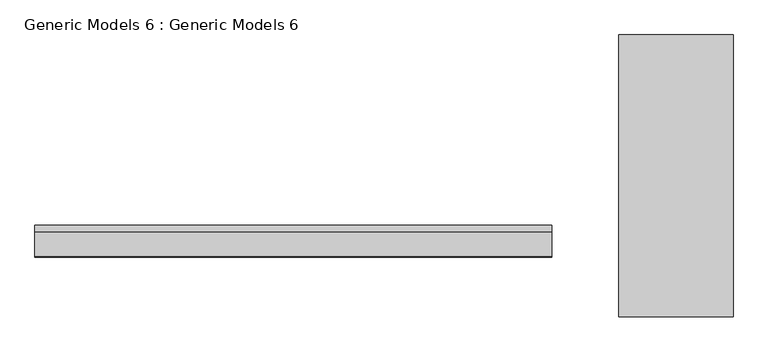
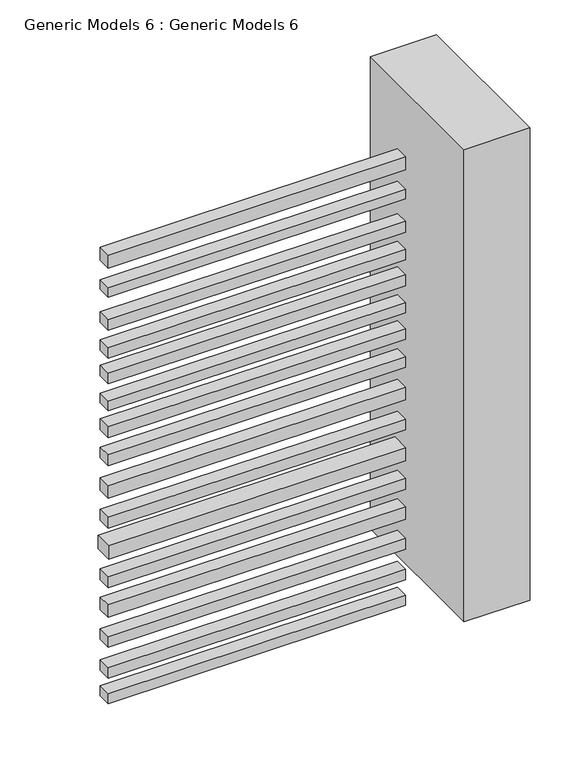
"""IFC4 building model written with IfcOpenShell, lengths in millimetres: proxy geometry, Generic Models 6 : Generic Models 6."""

from ifc_helpers import new_model, si_unit, frame, origin, place, context, project, spatial, polyline, outline, extrude, source, transform, mapped, element, save


def generic_models_6_generic_models_6_aa42e9c5(model_context):
    return source(origin(), model_context, "Body", "SweptSolid", [
        extrude(outline(polyline([(-872.4399578, -10539.5825842), (-872.4399578, -10641.1825842), (-2505.3020237, -10641.1825842), (-2505.3020237, -10539.5825842), (-872.4399578, -10539.5825842)])), frame((0.0, 0.0, 1201.0420271), z_axis=(0.0, 0.0, 1.0), x_axis=(1.0, 0.0, 0.0)), (0.0, 0.0, 1.0), 76.2),
        extrude(outline(polyline([(-872.4399578, -10562.4844889), (-872.4399578, -10638.6844889), (-2505.3020237, -10638.6844889), (-2505.3020237, -10562.4844889), (-872.4399578, -10562.4844889)])), frame((0.0, 0.0, 2889.4396101), z_axis=(0.0, 0.0, 1.0), x_axis=(1.0, 0.0, 0.0)), (0.0, 0.0, 1.0), 76.2),
        extrude(outline(polyline([(-872.4399578, -10562.4844889), (-872.4399578, -10638.6844889), (-2505.3020237, -10638.6844889), (-2505.3020237, -10562.4844889), (-872.4399578, -10562.4844889)])), frame((0.0, 0.0, 2721.6024053), z_axis=(0.0, 0.0, 1.0), x_axis=(1.0, 0.0, 0.0)), (0.0, 0.0, 1.0), 55.4181224),
        extrude(outline(polyline([(-872.4399578, -10562.4844889), (-872.4399578, -10638.6844889), (-2505.3020237, -10638.6844889), (-2505.3020237, -10562.4844889), (-872.4399578, -10562.4844889)])), frame((0.0, 0.0, 2528.0833777), z_axis=(0.0, 0.0, 1.0), x_axis=(1.0, 0.0, 0.0)), (0.0, 0.0, 1.0), 61.3490622),
        extrude(outline(polyline([(-872.4399578, -10562.4844889), (-872.4399578, -10638.6844889), (-2505.3020237, -10638.6844889), (-2505.3020237, -10562.4844889), (-872.4399578, -10562.4844889)])), frame((0.0, 0.0, 2366.3035704), z_axis=(0.0, 0.0, 1.0), x_axis=(1.0, 0.0, 0.0)), (0.0, 0.0, 1.0), 61.1302194),
        extrude(outline(polyline([(-872.4399578, -10562.4844889), (-872.4399578, -10638.6844889), (-2505.3020237, -10638.6844889), (-2505.3020237, -10562.4844889), (-872.4399578, -10562.4844889)])), frame((0.0, 0.0, 2217.3626191), z_axis=(0.0, 0.0, 1.0), x_axis=(1.0, 0.0, 0.0)), (0.0, 0.0, 1.0), 61.4127767),
        extrude(outline(polyline([(-872.4399578, -10562.4844889), (-872.4399578, -10638.6844889), (-2505.3020237, -10638.6844889), (-2505.3020237, -10562.4844889), (-872.4399578, -10562.4844889)])), frame((0.0, 0.0, 2060.4700214), z_axis=(0.0, 0.0, 1.0), x_axis=(1.0, 0.0, 0.0)), (0.0, 0.0, 1.0), 55.7215886),
        extrude(outline(polyline([(-872.4399578, -10562.4844889), (-872.4399578, -10638.6844889), (-2505.3020237, -10638.6844889), (-2505.3020237, -10562.4844889), (-872.4399578, -10562.4844889)])), frame((0.0, 0.0, 1905.0102311), z_axis=(0.0, 0.0, 1.0), x_axis=(1.0, 0.0, 0.0)), (0.0, 0.0, 1.0), 62.5430059),
        extrude(outline(polyline([(-872.4399578, -10562.4844889), (-872.4399578, -10638.6844889), (-2505.3020237, -10638.6844889), (-2505.3020237, -10562.4844889), (-872.4399578, -10562.4844889)])), frame((0.0, 0.0, 1742.9915599), z_axis=(0.0, 0.0, 1.0), x_axis=(1.0, 0.0, 0.0)), (0.0, 0.0, 1.0), 61.4127767),
        extrude(outline(polyline([(-872.4399578, -10562.4844889), (-872.4399578, -10638.6844889), (-2505.3020237, -10638.6844889), (-2505.3020237, -10562.4844889), (-872.4399578, -10562.4844889)])), frame((0.0, 0.0, 1553.7072405), z_axis=(0.0, 0.0, 1.0), x_axis=(1.0, 0.0, 0.0)), (0.0, 0.0, 1.0), 72.2100172),
        extrude(outline(polyline([(-872.4399578, -10562.4844889), (-872.4399578, -10638.6844889), (-2505.3020237, -10638.6844889), (-2505.3020237, -10562.4844889), (-872.4399578, -10562.4844889)])), frame((0.0, 0.0, 1378.0657556), z_axis=(0.0, 0.0, 1.0), x_axis=(1.0, 0.0, 0.0)), (0.0, 0.0, 1.0), 63.6532141),
        extrude(outline(polyline([(-872.4399578, -10562.4844889), (-872.4399578, -10638.6844889), (-2505.3020237, -10638.6844889), (-2505.3020237, -10562.4844889), (-872.4399578, -10562.4844889)])), frame((0.0, 0.0, 1032.9990467), z_axis=(0.0, 0.0, 1.0), x_axis=(1.0, 0.0, 0.0)), (0.0, 0.0, 1.0), 64.8234853),
        extrude(outline(polyline([(-872.4399578, -10562.4844889), (-872.4399578, -10638.6844889), (-2505.3020237, -10638.6844889), (-2505.3020237, -10562.4844889), (-872.4399578, -10562.4844889)])), frame((0.0, 0.0, 860.5508174), z_axis=(0.0, 0.0, 1.0), x_axis=(1.0, 0.0, 0.0)), (0.0, 0.0, 1.0), 72.4433357),
        extrude(outline(polyline([(-872.4399578, -10562.4844889), (-872.4399578, -10638.6844889), (-2505.3020237, -10638.6844889), (-2505.3020237, -10562.4844889), (-872.4399578, -10562.4844889)])), frame((0.0, 0.0, 686.3385598), z_axis=(0.0, 0.0, 1.0), x_axis=(1.0, 0.0, 0.0)), (0.0, 0.0, 1.0), 63.4936062),
        extrude(outline(polyline([(-872.4399578, -10562.4844889), (-872.4399578, -10638.6844889), (-2505.3020237, -10638.6844889), (-2505.3020237, -10562.4844889), (-872.4399578, -10562.4844889)])), frame((0.0, 0.0, 507.1252142), z_axis=(0.0, 0.0, 1.0), x_axis=(1.0, 0.0, 0.0)), (0.0, 0.0, 1.0), 61.0714053),
        extrude(outline(polyline([(-872.4399578, -10562.4844889), (-872.4399578, -10638.6844889), (-2505.3020237, -10638.6844889), (-2505.3020237, -10562.4844889), (-872.4399578, -10562.4844889)])), frame((0.0, 0.0, 360.0968631), z_axis=(0.0, 0.0, 1.0), x_axis=(1.0, 0.0, 0.0)), (0.0, 0.0, 1.0), 57.316237),
        extrude(outline(polyline([(-298.4695932, -10830.0220992), (-659.3229687, -10830.0220992), (-659.3229687, -9938.8923116), (-298.4695932, -9938.8923116), (-298.4695932, -10830.0220992)])), frame((0.0, 0.0, 304.8), z_axis=(0.0, 0.0, 1.0), x_axis=(1.0, 0.0, 0.0)), (0.0, 0.0, 1.0), 2743.2),
    ])


if __name__ == "__main__":
    model = new_model("IFC4")
    model_context = context("Model", 3, world=origin())
    ifc_project = project(units=[si_unit("LENGTHUNIT", "METRE", prefix="MILLI")], contexts=[model_context])
    site = spatial("IfcSite", under=ifc_project)
    building = spatial("IfcBuilding", under=site)
    placement = place(None, origin())
    generic_models_6_generic_models_6_shape = generic_models_6_generic_models_6_aa42e9c5(model_context)
    element("IfcBuildingElementProxy", 1, Name="Generic Models 6 : Generic Models 6", ObjectType="Generic Models 6 : Generic Models 6", at=placement, inside=building, context=model_context, shape_type="MappedRepresentation", body=[
        mapped(generic_models_6_generic_models_6_shape, transform((0.0, 0.0, 0.0), x_axis=(1.0, 0.0, 0.0), y_axis=(0.0, 1.0, 0.0), z_axis=(0.0, 0.0, 1.0))),
    ])
    save(model, "model.ifc")
